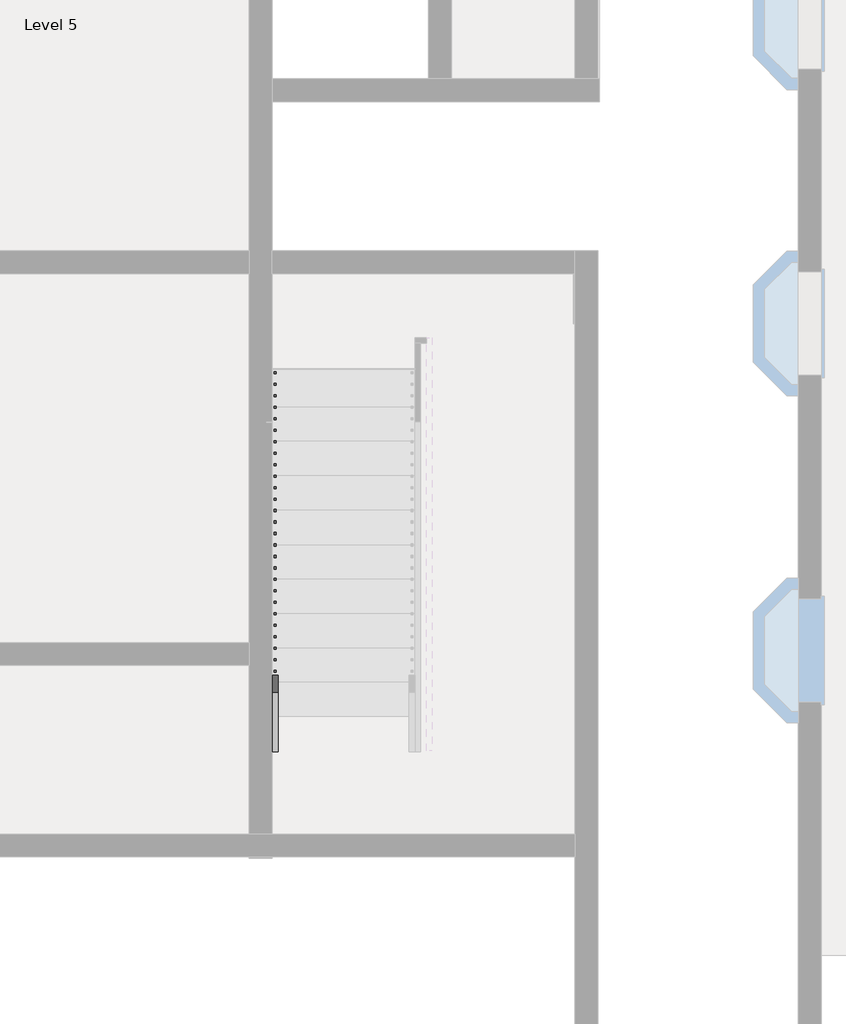
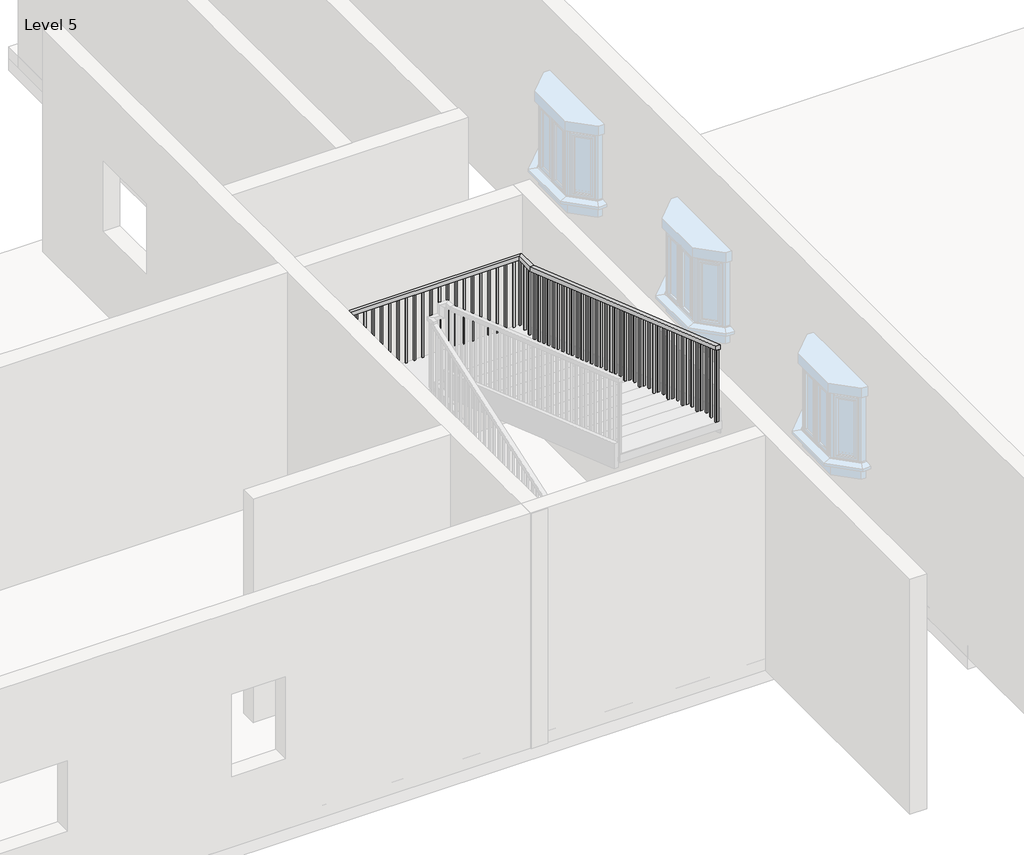
# One storey, part 8 of 14: 1 railing.
"""IFC4 building model written with IfcOpenShell, lengths in millimetres."""

from ifc_helpers import new_model, si_unit, frame, origin, place, context, project, spatial, polyline, outline, extrude, faceted_brep, element, save

model = new_model("IFC4")

# Units and contexts
model_context = context("Model", 3, world=origin())
ifc_project = project(units=[si_unit("LENGTHUNIT", "METRE", prefix="MILLI")], contexts=[model_context])

# Site, building, storey
site = spatial("IfcSite", under=ifc_project)
building = spatial("IfcBuilding", under=site)
storey = spatial("IfcBuildingStorey", under=building, Name="Level 5", Elevation=12192.0)

# Railing
placement = place(None, origin())
element("IfcRailing", 1, ObjectType="Handrail - Rectangular", at=placement, inside=storey, context=model_context, shape_type="SolidModel", body=[
    faceted_brep([(-3857.687215, -9955.5916506, 13211.9076923), (-3857.687215, -9955.5916506, 13158.1602476), (-3806.887215, -9955.5916506, 13158.1602476), (-3806.887215, -9955.5916506, 13211.9076923), (-3857.687215, -6291.6416506, 14478.0), (-3857.687215, -6283.1120276, 14427.2), (-3806.887215, -6283.1120276, 14427.2), (-3806.887215, -6291.6416506, 14478.0), (-3857.687215, -5713.7916506, 14478.0), (-3857.687215, -5713.7916506, 14427.2), (-3806.887215, -5764.5916506, 14427.2), (-3806.887215, -5764.5916506, 14478.0), (-1190.687215, -5713.7916506, 14478.0), (-1190.687215, -5713.7916506, 14427.2), (-1241.487215, -5764.5916506, 14427.2), (-1241.487215, -5764.5916506, 14478.0), (-1190.687215, -5986.8416506, 14478.0), (-1190.687215, -5995.3852679, 14427.2), (-1241.487215, -5995.3852679, 14427.2), (-1241.487215, -5986.8416506, 14478.0), (-1190.687215, -9949.2416506, 15849.6), (-1241.487215, -9949.2416506, 15849.6), (-1241.487215, -9949.2416506, 15795.842594), (-1190.687215, -9949.2416506, 15795.842594)], [[[0, 1, 2, 3]], [[1, 0, 4, 5]], [[2, 1, 5, 6]], [[3, 2, 6, 7]], [[0, 3, 7, 4]], [[5, 4, 8, 9]], [[6, 5, 9, 10]], [[7, 6, 10, 11]], [[4, 7, 11, 8]], [[9, 8, 12, 13]], [[10, 9, 13, 14]], [[11, 10, 14, 15]], [[8, 11, 15, 12]], [[13, 12, 16, 17]], [[14, 13, 17, 18]], [[15, 14, 18, 19]], [[12, 15, 19, 16]], [[20, 21, 22, 23]], [[17, 16, 20, 23]], [[18, 17, 23, 22]], [[19, 18, 22, 21]], [[16, 19, 21, 20]]]),
    extrude(outline(polyline([(-9895.2666506, 15777.1589402), (-9895.2666506, 14829.6923077), (-9914.3166506, 14829.6923077), (-9914.3166506, 15783.7531709), (-9895.2666506, 15777.1589402)])), frame((-1225.612215, 0.0, 0.0), z_axis=(1.0, 0.0, 0.0), x_axis=(0.0, 1.0, 0.0)), (0.0, 0.0, 1.0), 19.05),
    extrude(outline(polyline([(-9793.6666506, 15741.9897094), (-9793.6666506, 14829.6923077), (-9812.7166506, 14829.6923077), (-9812.7166506, 15748.5839402), (-9793.6666506, 15741.9897094)])), frame((-1225.612215, 0.0, 0.0), z_axis=(1.0, 0.0, 0.0), x_axis=(0.0, 1.0, 0.0)), (0.0, 0.0, 1.0), 19.05),
    extrude(outline(polyline([(-9692.0666506, 15706.8204786), (-9692.0666506, 14829.6923077), (-9711.1166506, 14829.6923077), (-9711.1166506, 15713.4147094), (-9692.0666506, 15706.8204786)])), frame((-1225.612215, 0.0, 0.0), z_axis=(1.0, 0.0, 0.0), x_axis=(0.0, 1.0, 0.0)), (0.0, 0.0, 1.0), 19.05),
    extrude(outline(polyline([(-9590.4666506, 15671.6512479), (-9590.4666506, 14724.1846154), (-9609.5166506, 14724.1846154), (-9609.5166506, 15678.2454786), (-9590.4666506, 15671.6512479)])), frame((-1225.612215, 0.0, 0.0), z_axis=(1.0, 0.0, 0.0), x_axis=(0.0, 1.0, 0.0)), (0.0, 0.0, 1.0), 19.05),
    extrude(outline(polyline([(-9488.8666506, 15636.4820171), (-9488.8666506, 14724.1846154), (-9507.9166506, 14724.1846154), (-9507.9166506, 15643.0762479), (-9488.8666506, 15636.4820171)])), frame((-1225.612215, 0.0, 0.0), z_axis=(1.0, 0.0, 0.0), x_axis=(0.0, 1.0, 0.0)), (0.0, 0.0, 1.0), 19.05),
    extrude(outline(polyline([(-9387.2666506, 15601.3127863), (-9387.2666506, 14724.1846154), (-9406.3166506, 14724.1846154), (-9406.3166506, 15607.9070171), (-9387.2666506, 15601.3127863)])), frame((-1225.612215, 0.0, 0.0), z_axis=(1.0, 0.0, 0.0), x_axis=(0.0, 1.0, 0.0)), (0.0, 0.0, 1.0), 19.05),
    extrude(outline(polyline([(-9285.6666506, 15566.1435556), (-9285.6666506, 14618.6769231), (-9304.7166506, 14618.6769231), (-9304.7166506, 15572.7377863), (-9285.6666506, 15566.1435556)])), frame((-1225.612215, 0.0, 0.0), z_axis=(1.0, 0.0, 0.0), x_axis=(0.0, 1.0, 0.0)), (0.0, 0.0, 1.0), 19.05),
    extrude(outline(polyline([(-9184.0666506, 15530.9743248), (-9184.0666506, 14618.6769231), (-9203.1166506, 14618.6769231), (-9203.1166506, 15537.5685556), (-9184.0666506, 15530.9743248)])), frame((-1225.612215, 0.0, 0.0), z_axis=(1.0, 0.0, 0.0), x_axis=(0.0, 1.0, 0.0)), (0.0, 0.0, 1.0), 19.05),
    extrude(outline(polyline([(-9082.4666506, 15495.805094), (-9082.4666506, 14618.6769231), (-9101.5166506, 14618.6769231), (-9101.5166506, 15502.3993248), (-9082.4666506, 15495.805094)])), frame((-1225.612215, 0.0, 0.0), z_axis=(1.0, 0.0, 0.0), x_axis=(0.0, 1.0, 0.0)), (0.0, 0.0, 1.0), 19.05),
    extrude(outline(polyline([(-8980.8666506, 15460.6358632), (-8980.8666506, 14513.1692308), (-8999.9166506, 14513.1692308), (-8999.9166506, 15467.230094), (-8980.8666506, 15460.6358632)])), frame((-1225.612215, 0.0, 0.0), z_axis=(1.0, 0.0, 0.0), x_axis=(0.0, 1.0, 0.0)), (0.0, 0.0, 1.0), 19.05),
    extrude(outline(polyline([(-8879.2666506, 15425.4666325), (-8879.2666506, 14513.1692308), (-8898.3166506, 14513.1692308), (-8898.3166506, 15432.0608632), (-8879.2666506, 15425.4666325)])), frame((-1225.612215, 0.0, 0.0), z_axis=(1.0, 0.0, 0.0), x_axis=(0.0, 1.0, 0.0)), (0.0, 0.0, 1.0), 19.05),
    extrude(outline(polyline([(-8777.6666506, 15390.2974017), (-8777.6666506, 14513.1692308), (-8796.7166506, 14513.1692308), (-8796.7166506, 15396.8916325), (-8777.6666506, 15390.2974017)])), frame((-1225.612215, 0.0, 0.0), z_axis=(1.0, 0.0, 0.0), x_axis=(0.0, 1.0, 0.0)), (0.0, 0.0, 1.0), 19.05),
    extrude(outline(polyline([(-8676.0666506, 15355.1281709), (-8676.0666506, 14407.6615385), (-8695.1166506, 14407.6615385), (-8695.1166506, 15361.7224017), (-8676.0666506, 15355.1281709)])), frame((-1225.612215, 0.0, 0.0), z_axis=(1.0, 0.0, 0.0), x_axis=(0.0, 1.0, 0.0)), (0.0, 0.0, 1.0), 19.05),
    extrude(outline(polyline([(-8574.4666506, 15319.9589402), (-8574.4666506, 14407.6615385), (-8593.5166506, 14407.6615385), (-8593.5166506, 15326.5531709), (-8574.4666506, 15319.9589402)])), frame((-1225.612215, 0.0, 0.0), z_axis=(1.0, 0.0, 0.0), x_axis=(0.0, 1.0, 0.0)), (0.0, 0.0, 1.0), 19.05),
    extrude(outline(polyline([(-8472.8666506, 15284.7897094), (-8472.8666506, 14407.6615385), (-8491.9166506, 14407.6615385), (-8491.9166506, 15291.3839402), (-8472.8666506, 15284.7897094)])), frame((-1225.612215, 0.0, 0.0), z_axis=(1.0, 0.0, 0.0), x_axis=(0.0, 1.0, 0.0)), (0.0, 0.0, 1.0), 19.05),
    extrude(outline(polyline([(-8371.2666506, 15249.6204786), (-8371.2666506, 14302.1538462), (-8390.3166506, 14302.1538462), (-8390.3166506, 15256.2147094), (-8371.2666506, 15249.6204786)])), frame((-1225.612215, 0.0, 0.0), z_axis=(1.0, 0.0, 0.0), x_axis=(0.0, 1.0, 0.0)), (0.0, 0.0, 1.0), 19.05),
    extrude(outline(polyline([(-8269.6666506, 15214.4512479), (-8269.6666506, 14302.1538462), (-8288.7166506, 14302.1538462), (-8288.7166506, 15221.0454786), (-8269.6666506, 15214.4512479)])), frame((-1225.612215, 0.0, 0.0), z_axis=(1.0, 0.0, 0.0), x_axis=(0.0, 1.0, 0.0)), (0.0, 0.0, 1.0), 19.05),
    extrude(outline(polyline([(-8168.0666506, 15179.2820171), (-8168.0666506, 14302.1538462), (-8187.1166506, 14302.1538462), (-8187.1166506, 15185.8762479), (-8168.0666506, 15179.2820171)])), frame((-1225.612215, 0.0, 0.0), z_axis=(1.0, 0.0, 0.0), x_axis=(0.0, 1.0, 0.0)), (0.0, 0.0, 1.0), 19.05),
    extrude(outline(polyline([(-8066.4666506, 15144.1127863), (-8066.4666506, 14196.6461538), (-8085.5166506, 14196.6461538), (-8085.5166506, 15150.7070171), (-8066.4666506, 15144.1127863)])), frame((-1225.612215, 0.0, 0.0), z_axis=(1.0, 0.0, 0.0), x_axis=(0.0, 1.0, 0.0)), (0.0, 0.0, 1.0), 19.05),
    extrude(outline(polyline([(-7964.8666506, 15108.9435556), (-7964.8666506, 14196.6461538), (-7983.9166506, 14196.6461538), (-7983.9166506, 15115.5377863), (-7964.8666506, 15108.9435556)])), frame((-1225.612215, 0.0, 0.0), z_axis=(1.0, 0.0, 0.0), x_axis=(0.0, 1.0, 0.0)), (0.0, 0.0, 1.0), 19.05),
    extrude(outline(polyline([(-7863.2666506, 15073.7743248), (-7863.2666506, 14196.6461538), (-7882.3166506, 14196.6461538), (-7882.3166506, 15080.3685556), (-7863.2666506, 15073.7743248)])), frame((-1225.612215, 0.0, 0.0), z_axis=(1.0, 0.0, 0.0), x_axis=(0.0, 1.0, 0.0)), (0.0, 0.0, 1.0), 19.05),
    extrude(outline(polyline([(-7761.6666506, 15038.605094), (-7761.6666506, 14091.1384615), (-7780.7166506, 14091.1384615), (-7780.7166506, 15045.1993248), (-7761.6666506, 15038.605094)])), frame((-1225.612215, 0.0, 0.0), z_axis=(1.0, 0.0, 0.0), x_axis=(0.0, 1.0, 0.0)), (0.0, 0.0, 1.0), 19.05),
    extrude(outline(polyline([(-7660.0666506, 15003.4358632), (-7660.0666506, 14091.1384615), (-7679.1166506, 14091.1384615), (-7679.1166506, 15010.030094), (-7660.0666506, 15003.4358632)])), frame((-1225.612215, 0.0, 0.0), z_axis=(1.0, 0.0, 0.0), x_axis=(0.0, 1.0, 0.0)), (0.0, 0.0, 1.0), 19.05),
    extrude(outline(polyline([(-7558.4666506, 14968.2666325), (-7558.4666506, 14091.1384615), (-7577.5166506, 14091.1384615), (-7577.5166506, 14974.8608632), (-7558.4666506, 14968.2666325)])), frame((-1225.612215, 0.0, 0.0), z_axis=(1.0, 0.0, 0.0), x_axis=(0.0, 1.0, 0.0)), (0.0, 0.0, 1.0), 19.05),
    extrude(outline(polyline([(-7456.8666506, 14933.0974017), (-7456.8666506, 13985.6307692), (-7475.9166506, 13985.6307692), (-7475.9166506, 14939.6916325), (-7456.8666506, 14933.0974017)])), frame((-1225.612215, 0.0, 0.0), z_axis=(1.0, 0.0, 0.0), x_axis=(0.0, 1.0, 0.0)), (0.0, 0.0, 1.0), 19.05),
    extrude(outline(polyline([(-7355.2666506, 14897.9281709), (-7355.2666506, 13985.6307692), (-7374.3166506, 13985.6307692), (-7374.3166506, 14904.5224017), (-7355.2666506, 14897.9281709)])), frame((-1225.612215, 0.0, 0.0), z_axis=(1.0, 0.0, 0.0), x_axis=(0.0, 1.0, 0.0)), (0.0, 0.0, 1.0), 19.05),
    extrude(outline(polyline([(-7253.6666506, 14862.7589402), (-7253.6666506, 13985.6307692), (-7272.7166506, 13985.6307692), (-7272.7166506, 14869.3531709), (-7253.6666506, 14862.7589402)])), frame((-1225.612215, 0.0, 0.0), z_axis=(1.0, 0.0, 0.0), x_axis=(0.0, 1.0, 0.0)), (0.0, 0.0, 1.0), 19.05),
    extrude(outline(polyline([(-7152.0666506, 14827.5897094), (-7152.0666506, 13880.1230769), (-7171.1166506, 13880.1230769), (-7171.1166506, 14834.1839402), (-7152.0666506, 14827.5897094)])), frame((-1225.612215, 0.0, 0.0), z_axis=(1.0, 0.0, 0.0), x_axis=(0.0, 1.0, 0.0)), (0.0, 0.0, 1.0), 19.05),
    extrude(outline(polyline([(-7050.4666506, 14792.4204786), (-7050.4666506, 13880.1230769), (-7069.5166506, 13880.1230769), (-7069.5166506, 14799.0147094), (-7050.4666506, 14792.4204786)])), frame((-1225.612215, 0.0, 0.0), z_axis=(1.0, 0.0, 0.0), x_axis=(0.0, 1.0, 0.0)), (0.0, 0.0, 1.0), 19.05),
    extrude(outline(polyline([(-6948.8666506, 14757.2512479), (-6948.8666506, 13880.1230769), (-6967.9166506, 13880.1230769), (-6967.9166506, 14763.8454786), (-6948.8666506, 14757.2512479)])), frame((-1225.612215, 0.0, 0.0), z_axis=(1.0, 0.0, 0.0), x_axis=(0.0, 1.0, 0.0)), (0.0, 0.0, 1.0), 19.05),
    extrude(outline(polyline([(-6847.2666506, 14722.0820171), (-6847.2666506, 13774.6153846), (-6866.3166506, 13774.6153846), (-6866.3166506, 14728.6762479), (-6847.2666506, 14722.0820171)])), frame((-1225.612215, 0.0, 0.0), z_axis=(1.0, 0.0, 0.0), x_axis=(0.0, 1.0, 0.0)), (0.0, 0.0, 1.0), 19.05),
    extrude(outline(polyline([(-6745.6666506, 14686.9127863), (-6745.6666506, 13774.6153846), (-6764.7166506, 13774.6153846), (-6764.7166506, 14693.5070171), (-6745.6666506, 14686.9127863)])), frame((-1225.612215, 0.0, 0.0), z_axis=(1.0, 0.0, 0.0), x_axis=(0.0, 1.0, 0.0)), (0.0, 0.0, 1.0), 19.05),
    extrude(outline(polyline([(-6644.0666506, 14651.7435556), (-6644.0666506, 13774.6153846), (-6663.1166506, 13774.6153846), (-6663.1166506, 14658.3377863), (-6644.0666506, 14651.7435556)])), frame((-1225.612215, 0.0, 0.0), z_axis=(1.0, 0.0, 0.0), x_axis=(0.0, 1.0, 0.0)), (0.0, 0.0, 1.0), 19.05),
    extrude(outline(polyline([(-6542.4666506, 14616.5743248), (-6542.4666506, 13669.1076923), (-6561.5166506, 13669.1076923), (-6561.5166506, 14623.1685556), (-6542.4666506, 14616.5743248)])), frame((-1225.612215, 0.0, 0.0), z_axis=(1.0, 0.0, 0.0), x_axis=(0.0, 1.0, 0.0)), (0.0, 0.0, 1.0), 19.05),
    extrude(outline(polyline([(-6440.8666506, 14581.405094), (-6440.8666506, 13669.1076923), (-6459.9166506, 13669.1076923), (-6459.9166506, 14587.9993248), (-6440.8666506, 14581.405094)])), frame((-1225.612215, 0.0, 0.0), z_axis=(1.0, 0.0, 0.0), x_axis=(0.0, 1.0, 0.0)), (0.0, 0.0, 1.0), 19.05),
    extrude(outline(polyline([(-6339.2666506, 14546.2358632), (-6339.2666506, 13669.1076923), (-6358.3166506, 13669.1076923), (-6358.3166506, 14552.830094), (-6339.2666506, 14546.2358632)])), frame((-1225.612215, 0.0, 0.0), z_axis=(1.0, 0.0, 0.0), x_axis=(0.0, 1.0, 0.0)), (0.0, 0.0, 1.0), 19.05),
    extrude(outline(polyline([(-6237.6666506, 14511.0666325), (-6237.6666506, 13563.6), (-6256.7166506, 13563.6), (-6256.7166506, 14517.6608632), (-6237.6666506, 14511.0666325)])), frame((-1225.612215, 0.0, 0.0), z_axis=(1.0, 0.0, 0.0), x_axis=(0.0, 1.0, 0.0)), (0.0, 0.0, 1.0), 19.05),
    extrude(outline(polyline([(-6136.0666506, 14475.8974017), (-6136.0666506, 13563.6), (-6155.1166506, 13563.6), (-6155.1166506, 14482.4916325), (-6136.0666506, 14475.8974017)])), frame((-1225.612215, 0.0, 0.0), z_axis=(1.0, 0.0, 0.0), x_axis=(0.0, 1.0, 0.0)), (0.0, 0.0, 1.0), 19.05),
    extrude(outline(polyline([(-6034.4666506, 14440.7281709), (-6034.4666506, 13563.6), (-6053.5166506, 13563.6), (-6053.5166506, 14447.3224017), (-6034.4666506, 14440.7281709)])), frame((-1225.612215, 0.0, 0.0), z_axis=(1.0, 0.0, 0.0), x_axis=(0.0, 1.0, 0.0)), (0.0, 0.0, 1.0), 19.05),
    extrude(outline(polyline([(-1206.562215, -5932.8666506), (-1206.562215, -5951.9166506), (-1225.612215, -5951.9166506), (-1225.612215, -5932.8666506), (-1206.562215, -5932.8666506)])), frame((0.0, 0.0, 13563.6), z_axis=(0.0, 0.0, 1.0), x_axis=(1.0, 0.0, 0.0)), (0.0, 0.0, 1.0), 863.6),
    extrude(outline(polyline([(-1206.562215, -5831.2666506), (-1206.562215, -5850.3166506), (-1225.612215, -5850.3166506), (-1225.612215, -5831.2666506), (-1206.562215, -5831.2666506)])), frame((0.0, 0.0, 13563.6), z_axis=(0.0, 0.0, 1.0), x_axis=(1.0, 0.0, 0.0)), (0.0, 0.0, 1.0), 863.6),
    extrude(outline(polyline([(-1301.812215, -5729.6666506), (-1282.762215, -5729.6666506), (-1282.762215, -5748.7166506), (-1301.812215, -5748.7166506), (-1301.812215, -5729.6666506)])), frame((0.0, 0.0, 13563.6), z_axis=(0.0, 0.0, 1.0), x_axis=(1.0, 0.0, 0.0)), (0.0, 0.0, 1.0), 863.6),
    extrude(outline(polyline([(-1403.412215, -5729.6666506), (-1384.362215, -5729.6666506), (-1384.362215, -5748.7166506), (-1403.412215, -5748.7166506), (-1403.412215, -5729.6666506)])), frame((0.0, 0.0, 13563.6), z_axis=(0.0, 0.0, 1.0), x_axis=(1.0, 0.0, 0.0)), (0.0, 0.0, 1.0), 863.6),
    extrude(outline(polyline([(-1505.012215, -5729.6666506), (-1485.962215, -5729.6666506), (-1485.962215, -5748.7166506), (-1505.012215, -5748.7166506), (-1505.012215, -5729.6666506)])), frame((0.0, 0.0, 13563.6), z_axis=(0.0, 0.0, 1.0), x_axis=(1.0, 0.0, 0.0)), (0.0, 0.0, 1.0), 863.6),
    extrude(outline(polyline([(-1606.612215, -5729.6666506), (-1587.562215, -5729.6666506), (-1587.562215, -5748.7166506), (-1606.612215, -5748.7166506), (-1606.612215, -5729.6666506)])), frame((0.0, 0.0, 13563.6), z_axis=(0.0, 0.0, 1.0), x_axis=(1.0, 0.0, 0.0)), (0.0, 0.0, 1.0), 863.6),
    extrude(outline(polyline([(-1708.212215, -5729.6666506), (-1689.162215, -5729.6666506), (-1689.162215, -5748.7166506), (-1708.212215, -5748.7166506), (-1708.212215, -5729.6666506)])), frame((0.0, 0.0, 13563.6), z_axis=(0.0, 0.0, 1.0), x_axis=(1.0, 0.0, 0.0)), (0.0, 0.0, 1.0), 863.6),
    extrude(outline(polyline([(-1809.812215, -5729.6666506), (-1790.762215, -5729.6666506), (-1790.762215, -5748.7166506), (-1809.812215, -5748.7166506), (-1809.812215, -5729.6666506)])), frame((0.0, 0.0, 13563.6), z_axis=(0.0, 0.0, 1.0), x_axis=(1.0, 0.0, 0.0)), (0.0, 0.0, 1.0), 863.6),
    extrude(outline(polyline([(-1911.412215, -5729.6666506), (-1892.362215, -5729.6666506), (-1892.362215, -5748.7166506), (-1911.412215, -5748.7166506), (-1911.412215, -5729.6666506)])), frame((0.0, 0.0, 13563.6), z_axis=(0.0, 0.0, 1.0), x_axis=(1.0, 0.0, 0.0)), (0.0, 0.0, 1.0), 863.6),
    extrude(outline(polyline([(-2013.012215, -5729.6666506), (-1993.962215, -5729.6666506), (-1993.962215, -5748.7166506), (-2013.012215, -5748.7166506), (-2013.012215, -5729.6666506)])), frame((0.0, 0.0, 13563.6), z_axis=(0.0, 0.0, 1.0), x_axis=(1.0, 0.0, 0.0)), (0.0, 0.0, 1.0), 863.6),
    extrude(outline(polyline([(-2114.612215, -5729.6666506), (-2095.562215, -5729.6666506), (-2095.562215, -5748.7166506), (-2114.612215, -5748.7166506), (-2114.612215, -5729.6666506)])), frame((0.0, 0.0, 13563.6), z_axis=(0.0, 0.0, 1.0), x_axis=(1.0, 0.0, 0.0)), (0.0, 0.0, 1.0), 863.6),
    extrude(outline(polyline([(-2216.212215, -5729.6666506), (-2197.162215, -5729.6666506), (-2197.162215, -5748.7166506), (-2216.212215, -5748.7166506), (-2216.212215, -5729.6666506)])), frame((0.0, 0.0, 13563.6), z_axis=(0.0, 0.0, 1.0), x_axis=(1.0, 0.0, 0.0)), (0.0, 0.0, 1.0), 863.6),
    extrude(outline(polyline([(-2317.812215, -5729.6666506), (-2298.762215, -5729.6666506), (-2298.762215, -5748.7166506), (-2317.812215, -5748.7166506), (-2317.812215, -5729.6666506)])), frame((0.0, 0.0, 13563.6), z_axis=(0.0, 0.0, 1.0), x_axis=(1.0, 0.0, 0.0)), (0.0, 0.0, 1.0), 863.6),
    extrude(outline(polyline([(-2419.412215, -5729.6666506), (-2400.362215, -5729.6666506), (-2400.362215, -5748.7166506), (-2419.412215, -5748.7166506), (-2419.412215, -5729.6666506)])), frame((0.0, 0.0, 13563.6), z_axis=(0.0, 0.0, 1.0), x_axis=(1.0, 0.0, 0.0)), (0.0, 0.0, 1.0), 863.6),
    extrude(outline(polyline([(-2521.012215, -5729.6666506), (-2501.962215, -5729.6666506), (-2501.962215, -5748.7166506), (-2521.012215, -5748.7166506), (-2521.012215, -5729.6666506)])), frame((0.0, 0.0, 13563.6), z_axis=(0.0, 0.0, 1.0), x_axis=(1.0, 0.0, 0.0)), (0.0, 0.0, 1.0), 863.6),
    extrude(outline(polyline([(-2622.612215, -5729.6666506), (-2603.562215, -5729.6666506), (-2603.562215, -5748.7166506), (-2622.612215, -5748.7166506), (-2622.612215, -5729.6666506)])), frame((0.0, 0.0, 13563.6), z_axis=(0.0, 0.0, 1.0), x_axis=(1.0, 0.0, 0.0)), (0.0, 0.0, 1.0), 863.6),
    extrude(outline(polyline([(-2724.212215, -5729.6666506), (-2705.162215, -5729.6666506), (-2705.162215, -5748.7166506), (-2724.212215, -5748.7166506), (-2724.212215, -5729.6666506)])), frame((0.0, 0.0, 13563.6), z_axis=(0.0, 0.0, 1.0), x_axis=(1.0, 0.0, 0.0)), (0.0, 0.0, 1.0), 863.6),
    extrude(outline(polyline([(-2825.812215, -5729.6666506), (-2806.762215, -5729.6666506), (-2806.762215, -5748.7166506), (-2825.812215, -5748.7166506), (-2825.812215, -5729.6666506)])), frame((0.0, 0.0, 13563.6), z_axis=(0.0, 0.0, 1.0), x_axis=(1.0, 0.0, 0.0)), (0.0, 0.0, 1.0), 863.6),
    extrude(outline(polyline([(-2927.412215, -5729.6666506), (-2908.362215, -5729.6666506), (-2908.362215, -5748.7166506), (-2927.412215, -5748.7166506), (-2927.412215, -5729.6666506)])), frame((0.0, 0.0, 13563.6), z_axis=(0.0, 0.0, 1.0), x_axis=(1.0, 0.0, 0.0)), (0.0, 0.0, 1.0), 863.6),
    extrude(outline(polyline([(-3029.012215, -5729.6666506), (-3009.962215, -5729.6666506), (-3009.962215, -5748.7166506), (-3029.012215, -5748.7166506), (-3029.012215, -5729.6666506)])), frame((0.0, 0.0, 13563.6), z_axis=(0.0, 0.0, 1.0), x_axis=(1.0, 0.0, 0.0)), (0.0, 0.0, 1.0), 863.6),
    extrude(outline(polyline([(-3130.612215, -5729.6666506), (-3111.562215, -5729.6666506), (-3111.562215, -5748.7166506), (-3130.612215, -5748.7166506), (-3130.612215, -5729.6666506)])), frame((0.0, 0.0, 13563.6), z_axis=(0.0, 0.0, 1.0), x_axis=(1.0, 0.0, 0.0)), (0.0, 0.0, 1.0), 863.6),
    extrude(outline(polyline([(-3232.212215, -5729.6666506), (-3213.162215, -5729.6666506), (-3213.162215, -5748.7166506), (-3232.212215, -5748.7166506), (-3232.212215, -5729.6666506)])), frame((0.0, 0.0, 13563.6), z_axis=(0.0, 0.0, 1.0), x_axis=(1.0, 0.0, 0.0)), (0.0, 0.0, 1.0), 863.6),
    extrude(outline(polyline([(-3333.812215, -5729.6666506), (-3314.762215, -5729.6666506), (-3314.762215, -5748.7166506), (-3333.812215, -5748.7166506), (-3333.812215, -5729.6666506)])), frame((0.0, 0.0, 13563.6), z_axis=(0.0, 0.0, 1.0), x_axis=(1.0, 0.0, 0.0)), (0.0, 0.0, 1.0), 863.6),
    extrude(outline(polyline([(-3435.412215, -5729.6666506), (-3416.362215, -5729.6666506), (-3416.362215, -5748.7166506), (-3435.412215, -5748.7166506), (-3435.412215, -5729.6666506)])), frame((0.0, 0.0, 13563.6), z_axis=(0.0, 0.0, 1.0), x_axis=(1.0, 0.0, 0.0)), (0.0, 0.0, 1.0), 863.6),
    extrude(outline(polyline([(-3537.012215, -5729.6666506), (-3517.962215, -5729.6666506), (-3517.962215, -5748.7166506), (-3537.012215, -5748.7166506), (-3537.012215, -5729.6666506)])), frame((0.0, 0.0, 13563.6), z_axis=(0.0, 0.0, 1.0), x_axis=(1.0, 0.0, 0.0)), (0.0, 0.0, 1.0), 863.6),
    extrude(outline(polyline([(-3638.612215, -5729.6666506), (-3619.562215, -5729.6666506), (-3619.562215, -5748.7166506), (-3638.612215, -5748.7166506), (-3638.612215, -5729.6666506)])), frame((0.0, 0.0, 13563.6), z_axis=(0.0, 0.0, 1.0), x_axis=(1.0, 0.0, 0.0)), (0.0, 0.0, 1.0), 863.6),
    extrude(outline(polyline([(-3740.212215, -5729.6666506), (-3721.162215, -5729.6666506), (-3721.162215, -5748.7166506), (-3740.212215, -5748.7166506), (-3740.212215, -5729.6666506)])), frame((0.0, 0.0, 13563.6), z_axis=(0.0, 0.0, 1.0), x_axis=(1.0, 0.0, 0.0)), (0.0, 0.0, 1.0), 863.6),
    extrude(outline(polyline([(-3841.812215, -5799.5166506), (-3841.812215, -5780.4666506), (-3822.762215, -5780.4666506), (-3822.762215, -5799.5166506), (-3841.812215, -5799.5166506)])), frame((0.0, 0.0, 13563.6), z_axis=(0.0, 0.0, 1.0), x_axis=(1.0, 0.0, 0.0)), (0.0, 0.0, 1.0), 863.6),
    extrude(outline(polyline([(-3841.812215, -5901.1166506), (-3841.812215, -5882.0666506), (-3822.762215, -5882.0666506), (-3822.762215, -5901.1166506), (-3841.812215, -5901.1166506)])), frame((0.0, 0.0, 13563.6), z_axis=(0.0, 0.0, 1.0), x_axis=(1.0, 0.0, 0.0)), (0.0, 0.0, 1.0), 863.6),
    extrude(outline(polyline([(-3841.812215, -6002.7166506), (-3841.812215, -5983.6666506), (-3822.762215, -5983.6666506), (-3822.762215, -6002.7166506), (-3841.812215, -6002.7166506)])), frame((0.0, 0.0, 13563.6), z_axis=(0.0, 0.0, 1.0), x_axis=(1.0, 0.0, 0.0)), (0.0, 0.0, 1.0), 863.6),
    extrude(outline(polyline([(-3841.812215, -6104.3166506), (-3841.812215, -6085.2666506), (-3822.762215, -6085.2666506), (-3822.762215, -6104.3166506), (-3841.812215, -6104.3166506)])), frame((0.0, 0.0, 13563.6), z_axis=(0.0, 0.0, 1.0), x_axis=(1.0, 0.0, 0.0)), (0.0, 0.0, 1.0), 863.6),
    extrude(outline(polyline([(-3841.812215, -6205.9166506), (-3841.812215, -6186.8666506), (-3822.762215, -6186.8666506), (-3822.762215, -6205.9166506), (-3841.812215, -6205.9166506)])), frame((0.0, 0.0, 13563.6), z_axis=(0.0, 0.0, 1.0), x_axis=(1.0, 0.0, 0.0)), (0.0, 0.0, 1.0), 863.6),
    extrude(outline(polyline([(-6288.4666506, 14425.349689), (-6288.4666506, 13458.0923077), (-6307.5166506, 13458.0923077), (-6307.5166506, 14418.7668867), (-6288.4666506, 14425.349689)])), frame((-3841.812215, 0.0, 0.0), z_axis=(1.0, 0.0, 0.0), x_axis=(0.0, 1.0, 0.0)), (0.0, 0.0, 1.0), 19.05),
    extrude(outline(polyline([(-6390.0666506, 14390.2414101), (-6390.0666506, 13458.0923077), (-6409.1166506, 13458.0923077), (-6409.1166506, 14383.6586078), (-6390.0666506, 14390.2414101)])), frame((-3841.812215, 0.0, 0.0), z_axis=(1.0, 0.0, 0.0), x_axis=(0.0, 1.0, 0.0)), (0.0, 0.0, 1.0), 19.05),
    extrude(outline(polyline([(-6491.6666506, 14355.1331312), (-6491.6666506, 13458.0923077), (-6510.7166506, 13458.0923077), (-6510.7166506, 14348.5503289), (-6491.6666506, 14355.1331312)])), frame((-3841.812215, 0.0, 0.0), z_axis=(1.0, 0.0, 0.0), x_axis=(0.0, 1.0, 0.0)), (0.0, 0.0, 1.0), 19.05),
    extrude(outline(polyline([(-6593.2666506, 14320.0248523), (-6593.2666506, 13352.5846154), (-6612.3166506, 13352.5846154), (-6612.3166506, 14313.44205), (-6593.2666506, 14320.0248523)])), frame((-3841.812215, 0.0, 0.0), z_axis=(1.0, 0.0, 0.0), x_axis=(0.0, 1.0, 0.0)), (0.0, 0.0, 1.0), 19.05),
    extrude(outline(polyline([(-6694.8666506, 14284.9165734), (-6694.8666506, 13352.5846154), (-6713.9166506, 13352.5846154), (-6713.9166506, 14278.3337711), (-6694.8666506, 14284.9165734)])), frame((-3841.812215, 0.0, 0.0), z_axis=(1.0, 0.0, 0.0), x_axis=(0.0, 1.0, 0.0)), (0.0, 0.0, 1.0), 19.05),
    extrude(outline(polyline([(-6796.4666506, 14249.8082945), (-6796.4666506, 13352.5846154), (-6815.5166506, 13352.5846154), (-6815.5166506, 14243.2254922), (-6796.4666506, 14249.8082945)])), frame((-3841.812215, 0.0, 0.0), z_axis=(1.0, 0.0, 0.0), x_axis=(0.0, 1.0, 0.0)), (0.0, 0.0, 1.0), 19.05),
    extrude(outline(polyline([(-6898.0666506, 14214.7000156), (-6898.0666506, 13247.0769231), (-6917.1166506, 13247.0769231), (-6917.1166506, 14208.1172133), (-6898.0666506, 14214.7000156)])), frame((-3841.812215, 0.0, 0.0), z_axis=(1.0, 0.0, 0.0), x_axis=(0.0, 1.0, 0.0)), (0.0, 0.0, 1.0), 19.05),
    extrude(outline(polyline([(-6999.6666506, 14179.5917367), (-6999.6666506, 13247.0769231), (-7018.7166506, 13247.0769231), (-7018.7166506, 14173.0089344), (-6999.6666506, 14179.5917367)])), frame((-3841.812215, 0.0, 0.0), z_axis=(1.0, 0.0, 0.0), x_axis=(0.0, 1.0, 0.0)), (0.0, 0.0, 1.0), 19.05),
    extrude(outline(polyline([(-7101.2666506, 14144.4834578), (-7101.2666506, 13247.0769231), (-7120.3166506, 13247.0769231), (-7120.3166506, 14137.9006556), (-7101.2666506, 14144.4834578)])), frame((-3841.812215, 0.0, 0.0), z_axis=(1.0, 0.0, 0.0), x_axis=(0.0, 1.0, 0.0)), (0.0, 0.0, 1.0), 19.05),
    extrude(outline(polyline([(-7202.8666506, 14109.375179), (-7202.8666506, 13141.5692308), (-7221.9166506, 13141.5692308), (-7221.9166506, 14102.7923767), (-7202.8666506, 14109.375179)])), frame((-3841.812215, 0.0, 0.0), z_axis=(1.0, 0.0, 0.0), x_axis=(0.0, 1.0, 0.0)), (0.0, 0.0, 1.0), 19.05),
    extrude(outline(polyline([(-7304.4666506, 14074.2669001), (-7304.4666506, 13141.5692308), (-7323.5166506, 13141.5692308), (-7323.5166506, 14067.6840978), (-7304.4666506, 14074.2669001)])), frame((-3841.812215, 0.0, 0.0), z_axis=(1.0, 0.0, 0.0), x_axis=(0.0, 1.0, 0.0)), (0.0, 0.0, 1.0), 19.05),
    extrude(outline(polyline([(-7406.0666506, 14039.1586212), (-7406.0666506, 13141.5692308), (-7425.1166506, 13141.5692308), (-7425.1166506, 14032.5758189), (-7406.0666506, 14039.1586212)])), frame((-3841.812215, 0.0, 0.0), z_axis=(1.0, 0.0, 0.0), x_axis=(0.0, 1.0, 0.0)), (0.0, 0.0, 1.0), 19.05),
    extrude(outline(polyline([(-7507.6666506, 14004.0503423), (-7507.6666506, 13036.0615385), (-7526.7166506, 13036.0615385), (-7526.7166506, 13997.46754), (-7507.6666506, 14004.0503423)])), frame((-3841.812215, 0.0, 0.0), z_axis=(1.0, 0.0, 0.0), x_axis=(0.0, 1.0, 0.0)), (0.0, 0.0, 1.0), 19.05),
    extrude(outline(polyline([(-7609.2666506, 13968.9420634), (-7609.2666506, 13036.0615385), (-7628.3166506, 13036.0615385), (-7628.3166506, 13962.3592611), (-7609.2666506, 13968.9420634)])), frame((-3841.812215, 0.0, 0.0), z_axis=(1.0, 0.0, 0.0), x_axis=(0.0, 1.0, 0.0)), (0.0, 0.0, 1.0), 19.05),
    extrude(outline(polyline([(-7710.8666506, 13933.8337845), (-7710.8666506, 13036.0615385), (-7729.9166506, 13036.0615385), (-7729.9166506, 13927.2509822), (-7710.8666506, 13933.8337845)])), frame((-3841.812215, 0.0, 0.0), z_axis=(1.0, 0.0, 0.0), x_axis=(0.0, 1.0, 0.0)), (0.0, 0.0, 1.0), 19.05),
    extrude(outline(polyline([(-7812.4666506, 13898.7255056), (-7812.4666506, 12930.5538462), (-7831.5166506, 12930.5538462), (-7831.5166506, 13892.1427033), (-7812.4666506, 13898.7255056)])), frame((-3841.812215, 0.0, 0.0), z_axis=(1.0, 0.0, 0.0), x_axis=(0.0, 1.0, 0.0)), (0.0, 0.0, 1.0), 19.05),
    extrude(outline(polyline([(-7914.0666506, 13863.6172267), (-7914.0666506, 12930.5538462), (-7933.1166506, 12930.5538462), (-7933.1166506, 13857.0344244), (-7914.0666506, 13863.6172267)])), frame((-3841.812215, 0.0, 0.0), z_axis=(1.0, 0.0, 0.0), x_axis=(0.0, 1.0, 0.0)), (0.0, 0.0, 1.0), 19.05),
    extrude(outline(polyline([(-8015.6666506, 13828.5089478), (-8015.6666506, 12930.5538462), (-8034.7166506, 12930.5538462), (-8034.7166506, 13821.9261455), (-8015.6666506, 13828.5089478)])), frame((-3841.812215, 0.0, 0.0), z_axis=(1.0, 0.0, 0.0), x_axis=(0.0, 1.0, 0.0)), (0.0, 0.0, 1.0), 19.05),
    extrude(outline(polyline([(-8117.2666506, 13793.4006689), (-8117.2666506, 12825.0461538), (-8136.3166506, 12825.0461538), (-8136.3166506, 13786.8178666), (-8117.2666506, 13793.4006689)])), frame((-3841.812215, 0.0, 0.0), z_axis=(1.0, 0.0, 0.0), x_axis=(0.0, 1.0, 0.0)), (0.0, 0.0, 1.0), 19.05),
    extrude(outline(polyline([(-8218.8666506, 13758.29239), (-8218.8666506, 12825.0461538), (-8237.9166506, 12825.0461538), (-8237.9166506, 13751.7095877), (-8218.8666506, 13758.29239)])), frame((-3841.812215, 0.0, 0.0), z_axis=(1.0, 0.0, 0.0), x_axis=(0.0, 1.0, 0.0)), (0.0, 0.0, 1.0), 19.05),
    extrude(outline(polyline([(-8320.4666506, 13723.1841111), (-8320.4666506, 12825.0461538), (-8339.5166506, 12825.0461538), (-8339.5166506, 13716.6013088), (-8320.4666506, 13723.1841111)])), frame((-3841.812215, 0.0, 0.0), z_axis=(1.0, 0.0, 0.0), x_axis=(0.0, 1.0, 0.0)), (0.0, 0.0, 1.0), 19.05),
    extrude(outline(polyline([(-8422.0666506, 13688.0758322), (-8422.0666506, 12719.5384615), (-8441.1166506, 12719.5384615), (-8441.1166506, 13681.4930299), (-8422.0666506, 13688.0758322)])), frame((-3841.812215, 0.0, 0.0), z_axis=(1.0, 0.0, 0.0), x_axis=(0.0, 1.0, 0.0)), (0.0, 0.0, 1.0), 19.05),
    extrude(outline(polyline([(-8523.6666506, 13652.9675533), (-8523.6666506, 12719.5384615), (-8542.7166506, 12719.5384615), (-8542.7166506, 13646.384751), (-8523.6666506, 13652.9675533)])), frame((-3841.812215, 0.0, 0.0), z_axis=(1.0, 0.0, 0.0), x_axis=(0.0, 1.0, 0.0)), (0.0, 0.0, 1.0), 19.05),
    extrude(outline(polyline([(-8625.2666506, 13617.8592744), (-8625.2666506, 12719.5384615), (-8644.3166506, 12719.5384615), (-8644.3166506, 13611.2764721), (-8625.2666506, 13617.8592744)])), frame((-3841.812215, 0.0, 0.0), z_axis=(1.0, 0.0, 0.0), x_axis=(0.0, 1.0, 0.0)), (0.0, 0.0, 1.0), 19.05),
    extrude(outline(polyline([(-8726.8666506, 13582.7509955), (-8726.8666506, 12614.0307692), (-8745.9166506, 12614.0307692), (-8745.9166506, 13576.1681932), (-8726.8666506, 13582.7509955)])), frame((-3841.812215, 0.0, 0.0), z_axis=(1.0, 0.0, 0.0), x_axis=(0.0, 1.0, 0.0)), (0.0, 0.0, 1.0), 19.05),
    extrude(outline(polyline([(-8828.4666506, 13547.6427166), (-8828.4666506, 12614.0307692), (-8847.5166506, 12614.0307692), (-8847.5166506, 13541.0599143), (-8828.4666506, 13547.6427166)])), frame((-3841.812215, 0.0, 0.0), z_axis=(1.0, 0.0, 0.0), x_axis=(0.0, 1.0, 0.0)), (0.0, 0.0, 1.0), 19.05),
    extrude(outline(polyline([(-8930.0666506, 13512.5344377), (-8930.0666506, 12614.0307692), (-8949.1166506, 12614.0307692), (-8949.1166506, 13505.9516354), (-8930.0666506, 13512.5344377)])), frame((-3841.812215, 0.0, 0.0), z_axis=(1.0, 0.0, 0.0), x_axis=(0.0, 1.0, 0.0)), (0.0, 0.0, 1.0), 19.05),
    extrude(outline(polyline([(-9031.6666506, 13477.4261588), (-9031.6666506, 12508.5230769), (-9050.7166506, 12508.5230769), (-9050.7166506, 13470.8433565), (-9031.6666506, 13477.4261588)])), frame((-3841.812215, 0.0, 0.0), z_axis=(1.0, 0.0, 0.0), x_axis=(0.0, 1.0, 0.0)), (0.0, 0.0, 1.0), 19.05),
    extrude(outline(polyline([(-9133.2666506, 13442.3178799), (-9133.2666506, 12508.5230769), (-9152.3166506, 12508.5230769), (-9152.3166506, 13435.7350776), (-9133.2666506, 13442.3178799)])), frame((-3841.812215, 0.0, 0.0), z_axis=(1.0, 0.0, 0.0), x_axis=(0.0, 1.0, 0.0)), (0.0, 0.0, 1.0), 19.05),
    extrude(outline(polyline([(-9234.8666506, 13407.209601), (-9234.8666506, 12508.5230769), (-9253.9166506, 12508.5230769), (-9253.9166506, 13400.6267987), (-9234.8666506, 13407.209601)])), frame((-3841.812215, 0.0, 0.0), z_axis=(1.0, 0.0, 0.0), x_axis=(0.0, 1.0, 0.0)), (0.0, 0.0, 1.0), 19.05),
    extrude(outline(polyline([(-9336.4666506, 13372.1013221), (-9336.4666506, 12403.0153846), (-9355.5166506, 12403.0153846), (-9355.5166506, 13365.5185198), (-9336.4666506, 13372.1013221)])), frame((-3841.812215, 0.0, 0.0), z_axis=(1.0, 0.0, 0.0), x_axis=(0.0, 1.0, 0.0)), (0.0, 0.0, 1.0), 19.05),
    extrude(outline(polyline([(-9438.0666506, 13336.9930432), (-9438.0666506, 12403.0153846), (-9457.1166506, 12403.0153846), (-9457.1166506, 13330.4102409), (-9438.0666506, 13336.9930432)])), frame((-3841.812215, 0.0, 0.0), z_axis=(1.0, 0.0, 0.0), x_axis=(0.0, 1.0, 0.0)), (0.0, 0.0, 1.0), 19.05),
    extrude(outline(polyline([(-9539.6666506, 13301.8847643), (-9539.6666506, 12403.0153846), (-9558.7166506, 12403.0153846), (-9558.7166506, 13295.301962), (-9539.6666506, 13301.8847643)])), frame((-3841.812215, 0.0, 0.0), z_axis=(1.0, 0.0, 0.0), x_axis=(0.0, 1.0, 0.0)), (0.0, 0.0, 1.0), 19.05),
    extrude(outline(polyline([(-9641.2666506, 13266.7764854), (-9641.2666506, 12297.5076923), (-9660.3166506, 12297.5076923), (-9660.3166506, 13260.1936831), (-9641.2666506, 13266.7764854)])), frame((-3841.812215, 0.0, 0.0), z_axis=(1.0, 0.0, 0.0), x_axis=(0.0, 1.0, 0.0)), (0.0, 0.0, 1.0), 19.05),
    extrude(outline(polyline([(-9742.8666506, 13231.6682065), (-9742.8666506, 12297.5076923), (-9761.9166506, 12297.5076923), (-9761.9166506, 13225.0854043), (-9742.8666506, 13231.6682065)])), frame((-3841.812215, 0.0, 0.0), z_axis=(1.0, 0.0, 0.0), x_axis=(0.0, 1.0, 0.0)), (0.0, 0.0, 1.0), 19.05),
    extrude(outline(polyline([(-9844.4666506, 13196.5599277), (-9844.4666506, 12297.5076923), (-9863.5166506, 12297.5076923), (-9863.5166506, 13189.9771254), (-9844.4666506, 13196.5599277)])), frame((-3841.812215, 0.0, 0.0), z_axis=(1.0, 0.0, 0.0), x_axis=(0.0, 1.0, 0.0)), (0.0, 0.0, 1.0), 19.05),
    extrude(outline(polyline([(-1225.612215, -5729.6666506), (-1206.562215, -5729.6666506), (-1206.562215, -5748.7166506), (-1225.612215, -5748.7166506), (-1225.612215, -5729.6666506)])), frame((0.0, 0.0, 13563.6), z_axis=(0.0, 0.0, 1.0), x_axis=(1.0, 0.0, 0.0)), (0.0, 0.0, 1.0), 863.6),
    extrude(outline(polyline([(-3841.812215, -5748.7166506), (-3841.812215, -5729.6666506), (-3822.762215, -5729.6666506), (-3822.762215, -5748.7166506), (-3841.812215, -5748.7166506)])), frame((0.0, 0.0, 13563.6), z_axis=(0.0, 0.0, 1.0), x_axis=(1.0, 0.0, 0.0)), (0.0, 0.0, 1.0), 863.6),
    extrude(outline(polyline([(-9930.1916506, 15789.2483632), (-9930.1916506, 14829.6923077), (-9949.2416506, 14829.6923077), (-9949.2416506, 15795.842594), (-9930.1916506, 15789.2483632)])), frame((-1225.612215, 0.0, 0.0), z_axis=(1.0, 0.0, 0.0), x_axis=(0.0, 1.0, 0.0)), (0.0, 0.0, 1.0), 19.05),
    extrude(outline(polyline([(-9936.5416506, 13164.7430499), (-9936.5416506, 12297.5076923), (-9955.5916506, 12297.5076923), (-9955.5916506, 13158.1602476), (-9936.5416506, 13164.7430499)])), frame((-3841.812215, 0.0, 0.0), z_axis=(1.0, 0.0, 0.0), x_axis=(0.0, 1.0, 0.0)), (0.0, 0.0, 1.0), 19.05),
])

save(model, "model.ifc")

# Revit data of these elements
# Type "Handrail - Rectangular"
#   Assembly Code = "C2010400"
#   built-in parameter 1008612 = 0.0416667 (stored number, unit not read)
#   built-in parameter 1008611 = 0.0416667 (stored number, unit not read)
#   built-in parameter 1008609 = 0.333333 (stored number, unit not read)
#   built-in parameter 1008604 = 0.166667 (stored number, unit not read)
#   built-in parameter 1008603 = 0.166667 (stored number, unit not read)
#   Railing Height = 3' - 0"
#   built-in parameter 1008630 = 2
#   built-in parameter 1008610 = 2
#   built-in parameter 1008618 = Baluster - Square : 3/4"
# Element 1 (IfcRailing, "Handrail - Rectangular")
#   Phase Created = New Construction
